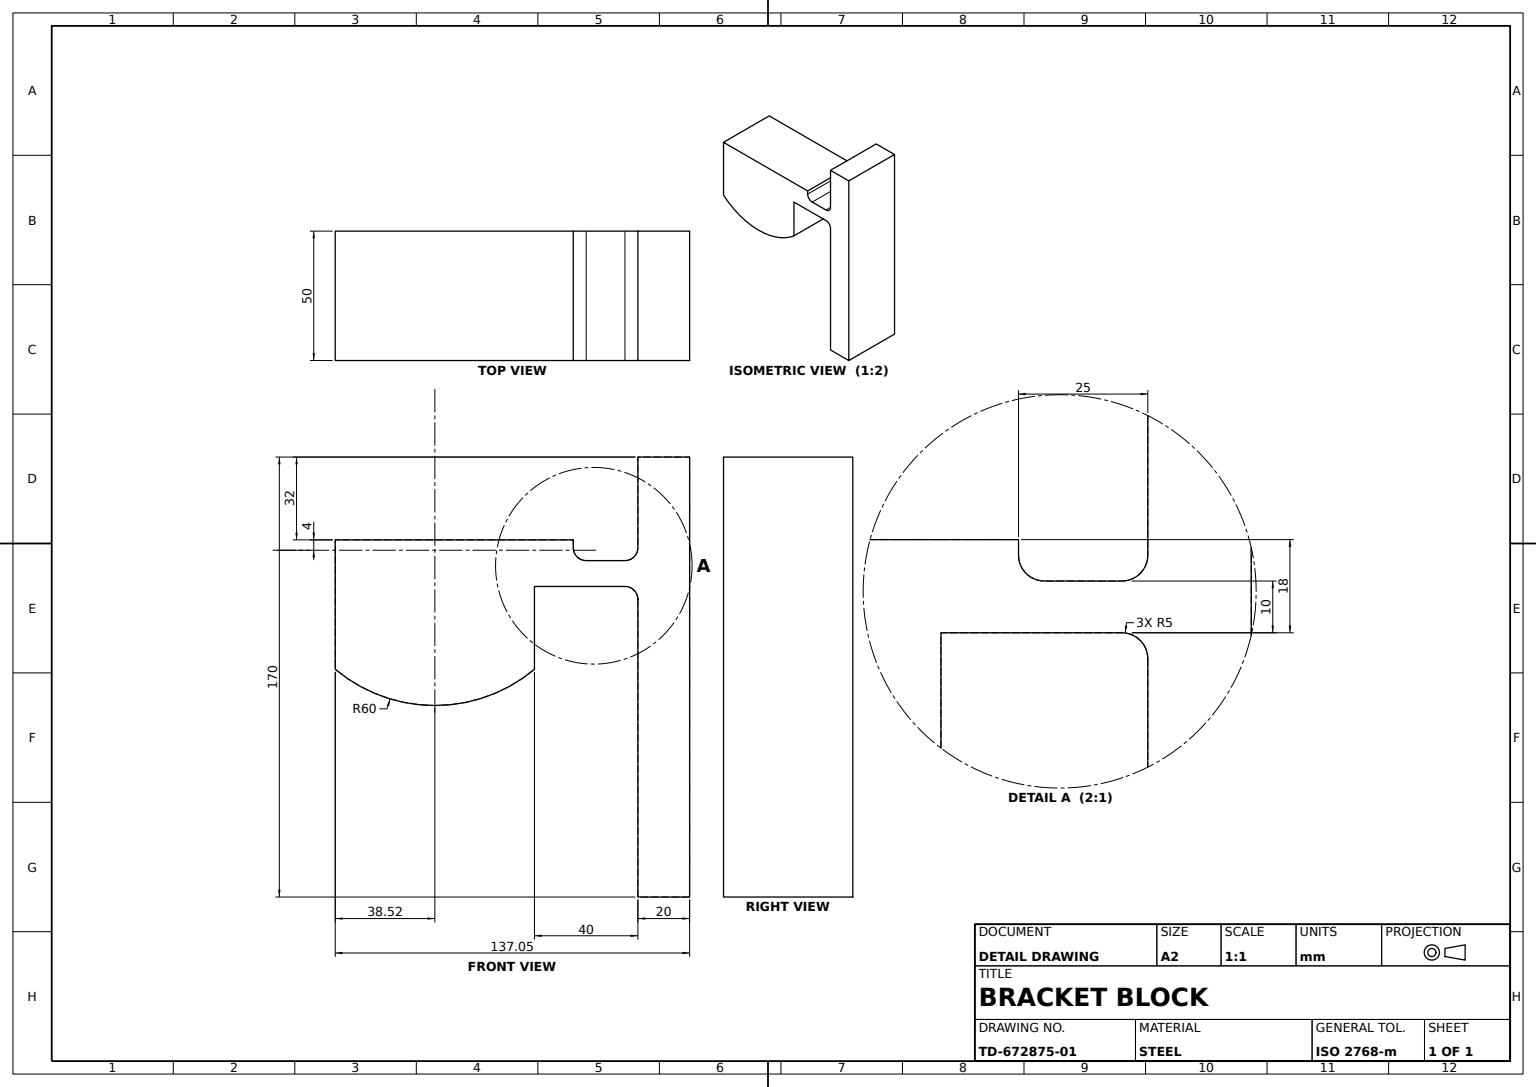
SolidWorks part; units mm, degrees
material "Plain Carbon Steel"
ref_plane "Front Plane" through (0, 0, 0) normal (0, 0, 1) x (1, 0, 0)
ref_plane "Top Plane" through (0, 0, 0) normal (0, 1, 0) x (1, 0, 0)
ref_plane "Right Plane" through (0, 0, 0) normal (1, 0, 0) x (0, 0, -1)
sketch "Back Plate Sketch" plane through (0, 0, 0) normal (1, 0, 0) x (0, 0, -1)
  line L1 (-10, 85) -> (10, 85)
  line L2 (-10, 85) -> (-10, -85)
  line L3 (-10, -85) -> (10, -85)
  line L4 (10, 85) -> (10, -85)
  line L5 (-10, 85) -> (10, -85) construction
  line L6 (-10, -85) -> (10, 85) construction
  point P0 (0, 0)
  dimension "D1" = 170
  dimension "D2" = 20
extrude "Back Plate" add sketch "Back Plate Sketch" along normal mid plane 50
sketch "Neck Boss Sketch" plane through (25, 0, 0) normal (1, 0, 0) x (0, 0, -1)
  line L1 (-10, 85) -> (-10, -85) construction
  line L3 (-30, 45) -> (-10, 45)
  line L4 (-10, 45) -> (-10, 35)
  line L5 (10, 85) -> (-10, 85) construction
  line L6 (-35, 50) -> (-35, 53)
  line L7 (-35, 53) -> (-50, 53)
  line L8 (-50, 53) -> (-50, 35)
  line L9 (-50, 35) -> (-10, 35)
  arc A0 (-30, 45) -> (-35, 50) centre (-30, 50) cw
  dimension "D3" = 5
  dimension "D1" = 40
  dimension "D2" = 10
  dimension "D4" = 15
  dimension "D5" = 20
  dimension "D6" = 18
extrude "Neck Boss" add sketch "Neck Boss Sketch" against normal through all contours L8 L9 L4 L3 A0 L6 L7
fillet "Neck Fillet R5" radius 5 2 edges at (0, 35, 10) (0, 45, 10)
sketch "Arm Block Sketch" plane through (25, 0, 0) normal (1, 0, 0) x (0, 0, -1)
  line L0 (-42.5, 49) -> (-142.5, 49) construction
  line L2 (-35, 53) -> (-50, 53) construction
  line L5 (-50, 53) -> (-50, 3)
  line L7 (-127.0454, 53) -> (-50, 53)
  line L8 (-127.0454, 3) -> (-127.0454, 53)
  line L9 (-50, 53) -> (-50, 35) construction
  arc A1 (-127.0454, 3) -> (-50, 3) centre (-88.5227, 49) ccw
  dimension "D6" = 50
  dimension "D3" = 60
  dimension "D1" = 100
  dimension "D2" = 4
  dimension "D5" = 50
extrude "Arm Block" add sketch "Arm Block Sketch" against normal through all
